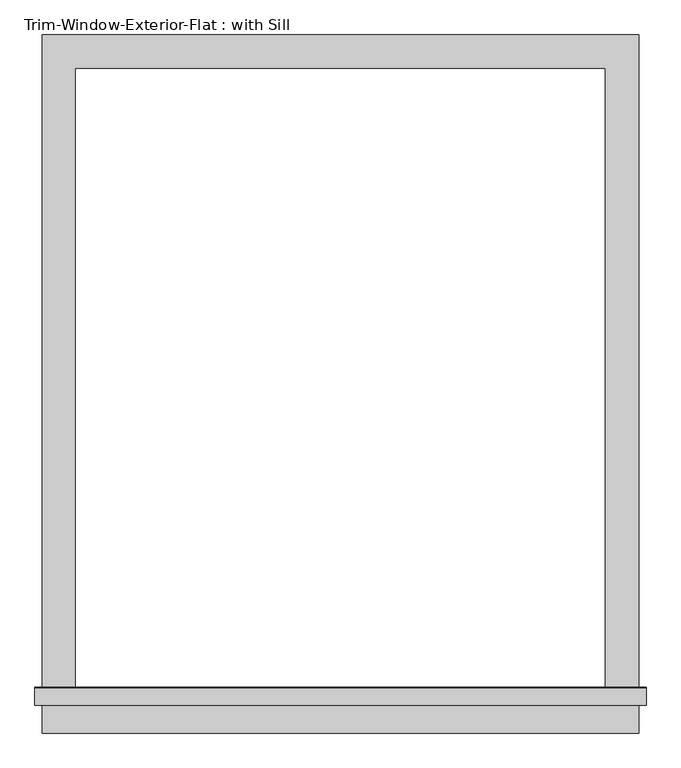
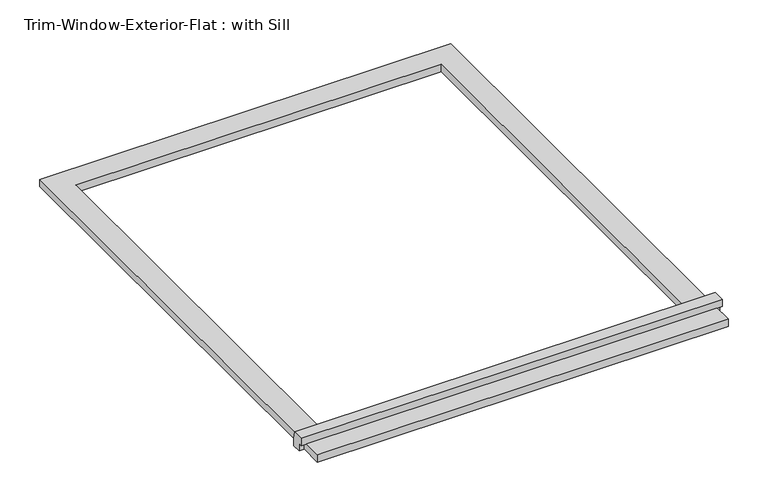
"""IFC4 building model written with IfcOpenShell, lengths in millimetres: proxy geometry, Trim-Window-Exterior-Flat : with Sill."""

from ifc_helpers import new_model, si_unit, frame, origin, origin_with_axes, place, context, project, spatial, polyline, outline, extrude, source, transform, mapped, element, save


def trim_window_exterior_flat_with_sill_1a1a26d5(model_context):
    return source(origin(), model_context, "Body", "SweptSolid", [
        extrude(outline(polyline([(514.35, -1088.9823709), (514.35, -1146.1323709), (-514.35, -1146.1323709), (-514.35, -1088.9823709), (514.35, -1088.9823709)])), origin_with_axes(), (0.0, 0.0, 1.0), 19.05),
        extrude(outline(polyline([(-1098.55, 38.1), (-1069.2580645, 38.1), (-1066.8, 19.05), (-1066.8, 0.0), (-1088.9823709, 0.0), (-1088.9823709, 19.05), (-1098.55, 19.05), (-1098.55, 38.1)])), frame((-527.05, 0.0, 0.0), z_axis=(1.0, 0.0, 0.0), x_axis=(0.0, 1.0, 0.0)), (0.0, 0.0, 1.0), 1054.1),
        extrude(outline(polyline([(-514.35, 57.15), (514.35, 57.15), (514.35, -1066.8), (457.2, -1066.8), (457.2, 0.0), (-457.2, 0.0), (-457.2, -1066.8), (-514.35, -1066.8), (-514.35, 57.15)])), origin_with_axes(), (0.0, 0.0, 1.0), 19.05),
    ])


if __name__ == "__main__":
    model = new_model("IFC4")
    model_context = context("Model", 3, world=origin())
    ifc_project = project(units=[si_unit("LENGTHUNIT", "METRE", prefix="MILLI")], contexts=[model_context])
    site = spatial("IfcSite", under=ifc_project)
    building = spatial("IfcBuilding", under=site)
    placement = place(None, origin())
    trim_window_exterior_flat_with_sill_shape = trim_window_exterior_flat_with_sill_1a1a26d5(model_context)
    element("IfcBuildingElementProxy", 1, Name="Trim-Window-Exterior-Flat : with Sill", ObjectType="Trim-Window-Exterior-Flat : with Sill", at=placement, inside=building, context=model_context, shape_type="MappedRepresentation", body=[
        mapped(trim_window_exterior_flat_with_sill_shape, transform((0.0, 0.0, 0.0), x_axis=(1.0, 0.0, 0.0), y_axis=(0.0, 1.0, 0.0), z_axis=(0.0, 0.0, 1.0))),
    ])
    save(model, "model.ifc")

# Revit data of these elements
# Type "Trim-Window-Exterior-Flat : with Sill"
#   Trim Width = 0' - 2 1/4"
#   Trim Thickness_Picture Frame = 0' - 1 1/4"
#   Trim Thickness_with Sill = 0' - 0 3/4"
#   Sill Thickness = 0' - 1 1/4"
#   Opening Width [instance default] = 2' - 0"
#   Opening Height [instance default] = 3' - 0"
#   Default Elevation = 4' - 0"
#   Sill = yes
#   Picture Frame = no
#   Trim Material [instance default] = none
# Element 1 (IfcBuildingElementProxy, "Trim-Window-Exterior-Flat : with Sill")
#   Opening Width = 3' - 0"
#   Opening Height = 3' - 6"
#   Trim Material = Clad - White
#   Materials on its faces: "Clad - White"
# Materials
#   "Clad - White": class "Wood", colour RGB 242 242 238, transparency 0, Cost = 0
